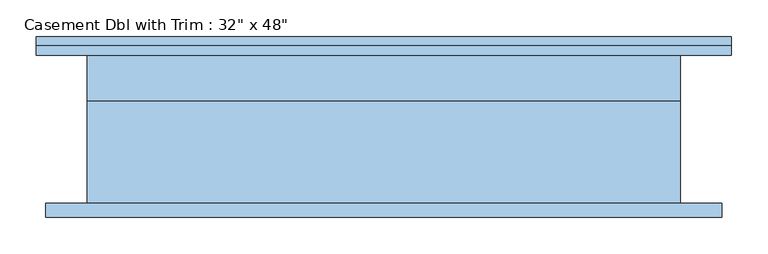
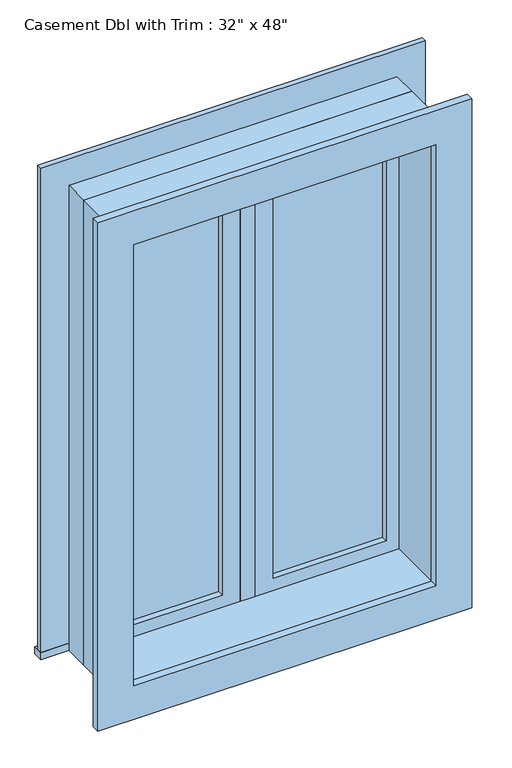
"""IFC4 building model written with IfcOpenShell, lengths in millimetres: window geometry."""

from ifc_helpers import new_model, si_unit, frame, origin, place, context, project, spatial, polyline, outline, extrude, source, transform, mapped, element, save


def window_bb17773d(model_context):
    return source(origin(), model_context, "Body", "SweptSolid", [
        extrude(outline(polyline([(63.5, 85.725), (342.9, 85.725), (342.9, 73.025), (63.5, 73.025), (63.5, 85.725)])), frame((0.0, 0.0, 977.9), z_axis=(0.0, 0.0, 1.0), x_axis=(1.0, 0.0, 0.0)), (0.0, 0.0, 1.0), 1092.2),
        extrude(outline(polyline([(2114.55, 19.05), (933.45, 19.05), (933.45, 387.35), (2114.55, 387.35), (2114.55, 19.05)]), holes=[polyline([(2070.1, 63.5), (2070.1, 342.9), (977.9, 342.9), (977.9, 63.5), (2070.1, 63.5)])]), frame((0.0, 57.15, 0.0), z_axis=(0.0, 1.0, 0.0), x_axis=(0.0, 0.0, 1.0)), (0.0, 0.0, 1.0), 44.45),
        extrude(outline(polyline([(19.05, 57.15), (-19.05, 57.15), (-19.05, 120.65), (19.05, 120.65), (19.05, 57.15)])), frame((0.0, 0.0, 933.45), z_axis=(0.0, 0.0, 1.0), x_axis=(1.0, 0.0, 0.0)), (0.0, 0.0, 1.0), 1181.1),
        extrude(outline(polyline([(-476.25, 146.05), (476.25, 146.05), (476.25, 120.65), (-476.25, 120.65), (-476.25, 146.05)])), frame((0.0, 0.0, 914.4), z_axis=(0.0, 0.0, 1.0), x_axis=(1.0, 0.0, 0.0)), (0.0, 0.0, 1.0), 19.05),
        extrude(outline(polyline([(2114.55, -387.35), (2114.55, 387.35), (933.45, 387.35), (933.45, 476.25), (2203.45, 476.25), (2203.45, -476.25), (933.45, -476.25), (933.45, -387.35), (2114.55, -387.35)])), frame((0.0, 120.65, 0.0), z_axis=(0.0, 1.0, 0.0), x_axis=(0.0, 0.0, 1.0)), (0.0, 0.0, 1.0), 12.7),
        extrude(outline(polyline([(2190.75, 463.55), (2190.75, -463.55), (857.25, -463.55), (857.25, 463.55), (2190.75, 463.55)]), holes=[polyline([(2101.85, 374.65), (946.15, 374.65), (946.15, -374.65), (2101.85, -374.65), (2101.85, 374.65)])]), frame((0.0, -101.6, 0.0), z_axis=(0.0, 1.0, 0.0), x_axis=(0.0, 0.0, 1.0)), (0.0, 0.0, 1.0), 19.05),
        extrude(outline(polyline([(-63.5, 73.025), (-342.9, 73.025), (-342.9, 85.725), (-63.5, 85.725), (-63.5, 73.025)])), frame((0.0, 0.0, 977.9), z_axis=(0.0, 0.0, 1.0), x_axis=(1.0, 0.0, 0.0)), (0.0, 0.0, 1.0), 1092.2),
        extrude(outline(polyline([(2114.55, -387.35), (933.45, -387.35), (933.45, -19.05), (2114.55, -19.05), (2114.55, -387.35)]), holes=[polyline([(2070.1, -342.9), (2070.1, -63.5), (977.9, -63.5), (977.9, -342.9), (2070.1, -342.9)])]), frame((0.0, 57.15, 0.0), z_axis=(0.0, 1.0, 0.0), x_axis=(0.0, 0.0, 1.0)), (0.0, 0.0, 1.0), 44.45),
        extrude(outline(polyline([(2133.6, -406.4), (914.4, -406.4), (914.4, 406.4), (2133.6, 406.4), (2133.6, -406.4)]), holes=[polyline([(2101.85, -374.65), (2101.85, 374.65), (946.15, 374.65), (946.15, -374.65), (2101.85, -374.65)])]), frame((0.0, -82.55, 0.0), z_axis=(0.0, 1.0, 0.0), x_axis=(0.0, 0.0, 1.0)), (0.0, 0.0, 1.0), 139.7),
        extrude(outline(polyline([(2133.6, 406.4), (2133.6, -406.4), (914.4, -406.4), (914.4, 406.4), (2133.6, 406.4)]), holes=[polyline([(2114.55, 387.35), (933.45, 387.35), (933.45, -387.35), (2114.55, -387.35), (2114.55, 387.35)])]), frame((0.0, 57.15, 0.0), z_axis=(0.0, 1.0, 0.0), x_axis=(0.0, 0.0, 1.0)), (0.0, 0.0, 1.0), 63.5),
    ])


if __name__ == "__main__":
    model = new_model("IFC4")
    model_context = context("Model", 3, world=origin())
    ifc_project = project(units=[si_unit("LENGTHUNIT", "METRE", prefix="MILLI")], contexts=[model_context])
    site = spatial("IfcSite", under=ifc_project)
    building = spatial("IfcBuilding", under=site)
    placement = place(None, origin())
    window_shape = window_bb17773d(model_context)
    element("IfcWindow", 1, ObjectType="Casement Dbl with Trim : 32\" x 48\"", at=placement, inside=building, context=model_context, shape_type="MappedRepresentation", body=[
        mapped(window_shape, transform((0.0, 0.0, 0.0), x_axis=(1.0, 0.0, 0.0), y_axis=(0.0, 1.0, 0.0), z_axis=(0.0, 0.0, 1.0))),
    ])
    save(model, "model.ifc")

# Revit data of these elements
# Type "Casement Dbl with Trim : 32\" x 48\""
#   Type Mark = "19"
#   Construction Type Id = "GSP4R"
#   Assembly Code = "B2020100"
#   Analytic Construction = "1/8 in Pilkington single glazing"
#   Visual Light Transmittance = 0.9
#   Solar Heat Gain Coefficient = 0.78
#   Heat Transfer Coefficient (U) = 0.6496 BTU/(h·ft²·°F)
#   Height = 4' - 0"
#   Default Sill Height = 3' - 0"
#   Trim Projection - Ext. = 0' - 0 1/2"
#   Trim Projection - Int. = 0' - 0 3/4"
#   Trim Width - Exterior = 0' - 3 1/2"
#   Trim Width - Interior = 0' - 3 1/2"
#   Width = 2' - 8"
#   Window Inset = 0' - 0 3/4"
#   Define Thermal Properties by = 1
#   Glass Pane Material = Glass
#   Sash Material = Sash
#   Trim Exterior Material = Trim
#   Trim Interior Material = Trim
#   Wall Closure = (empty or 0)
# Element 1 (IfcWindow, "Casement Dbl with Trim : 32\" x 48\"")
#   Materials on its faces: "Sash", "Trim", "Glass"
# Materials
#   "Glass": class "Glass", colour RGB 0 128 192, transparency 0.75, Description = "Soda Lime Glass", Cost = 0
#   "Sash": class "Wood", colour RGB 224 178 126, transparency 0
#   "Trim": class "Wood", colour RGB 224 178 126, transparency 0
